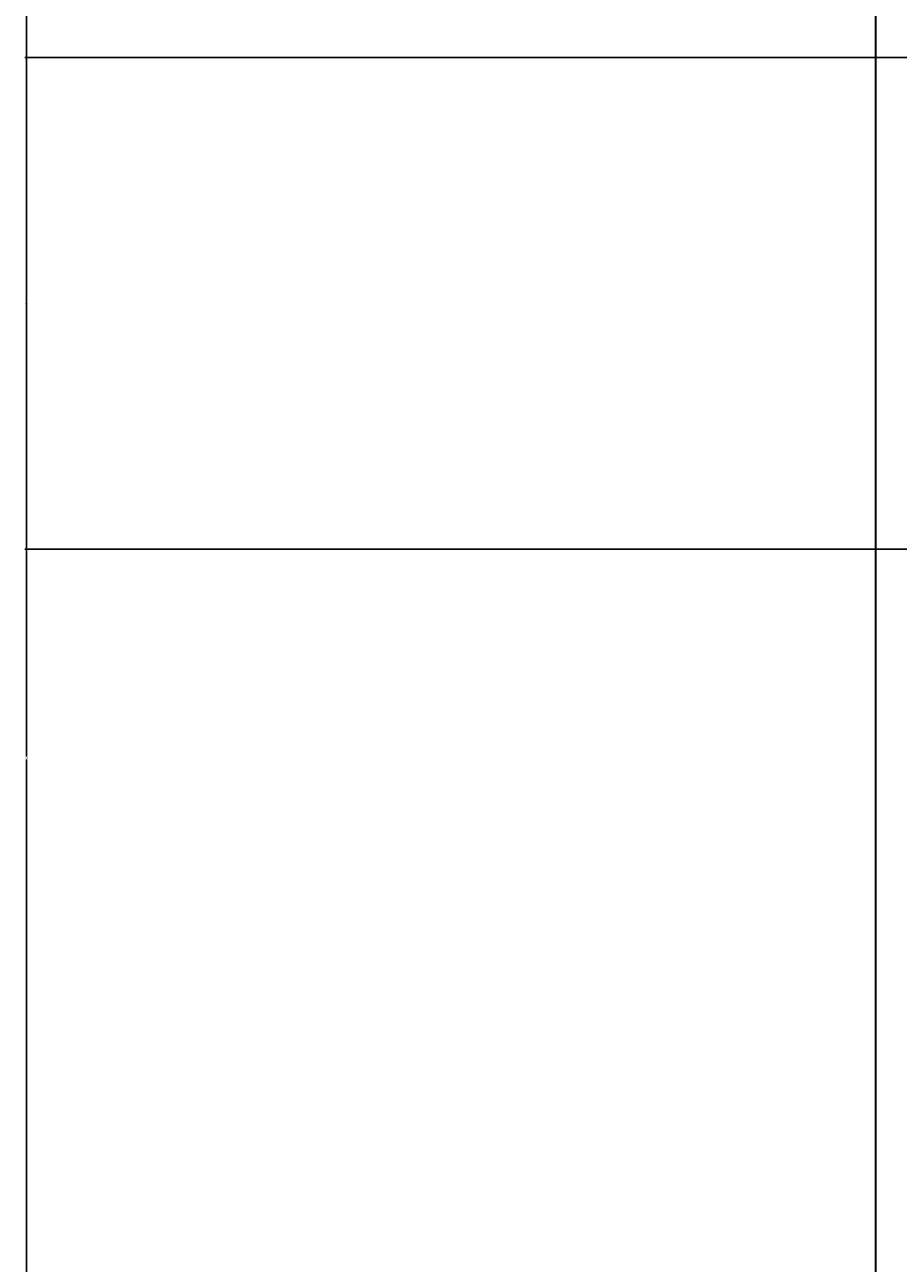
# Model space of a CAD drawing. Units: inches. Extents: x 3731 to 4318, y 1310 to 2388.
# Tile 24 of 57: x 3731 to 3838, y 1787 to 1938. Entities that reach past the tile are written whole.
import ezdxf

# ---------------------------------------------------------------- set-up
doc = ezdxf.new("R2010")
doc.units = ezdxf.units.IN
doc.layers.add('A-ANNO-DIMS', color=2, linetype='Continuous', lineweight=18)
doc.layers.add('A-WALL', color=7, linetype='Continuous', lineweight=35)
doc.styles.get("Standard").update_dxf_attribs({"font": 'arial.ttf'})
doc.dimstyles.get("Standard").update_dxf_attribs({"dimtxt": 0.18, "dimasz": 0.18, "dimexe": 0.18, "dimexo": 0.0625, "dimgap": 0.09, "dimtad": 0, "dimtih": 1, "dimtoh": 1, "dimdec": 4, "dimzin": 0, "dimdsep": 46, "dimtxsty": 'Standard', "dimcen": 0.09, "dimadec": 0, "dimazin": 0, "dimtfac": 1, "dimtdec": 4, "dimtofl": 0, "dimtmove": 0, "dimatfit": 3, "dimfxl": 1, "dimtolj": 1, "dimtzin": 0, "dimarcsym": 0})

# ---------------------------------------------------------------- blocks, each defined once
blk = doc.blocks.new('*D33')
at = {"layer": 'A-ANNO-DIMS', "color": 0, "lineweight": -2, "transparency": 16777216}
for p, q in [((3835.15, 2338.38), (3731.41, 2338.38)), ((3731.59, 2338.2), (3731.59, 1849.06)), ((3731.59, 1359.56), (3731.59, 1848.7)), ((3835.15, 1359.38), (3731.41, 1359.38))]:
    blk.add_line(p, q, dxfattribs=at)
at = {"layer": 'A-ANNO-DIMS', "color": 0, "transparency": 16777216}
for points in [[(3731.56, 2338.2), (3731.62, 2338.2), (3731.59, 2338.38)], [(3731.56, 1359.56), (3731.62, 1359.56), (3731.59, 1359.38)]]:
    blk.add_solid(points, dxfattribs=at)
at = {"layer": 'Defpoints', "color": 0, "transparency": 16777216}
for p in [(3731.59, 2338.38), (3835.21, 2338.38), (3835.21, 1359.38)]:
    blk.add_point(p, dxfattribs=at)
at = {"layer": 'A-ANNO-DIMS', "color": 0, "transparency": 16777216, "insert": (3731.59, 1848.88), "char_height": 0.18, "attachment_point": 5}
blk.add_mtext('\\A1;979', dxfattribs=at)
blk = doc.blocks.new('*D45')
at = {"layer": 'A-ANNO-DIMS', "color": 0, "lineweight": -2, "transparency": 16777216}
for p, q in [((3969.15, 1934.38), (3731.41, 1934.38)), ((3731.59, 1934.2), (3731.59, 1904.56)), ((3731.59, 1874.56), (3731.59, 1904.2)), ((3969.15, 1874.38), (3731.41, 1874.38))]:
    blk.add_line(p, q, dxfattribs=at)
at = {"layer": 'A-ANNO-DIMS', "color": 0, "transparency": 16777216}
for points in [[(3731.56, 1934.2), (3731.62, 1934.2), (3731.59, 1934.38)], [(3731.56, 1874.56), (3731.62, 1874.56), (3731.59, 1874.38)]]:
    blk.add_solid(points, dxfattribs=at)
at = {"layer": 'Defpoints', "color": 0, "transparency": 16777216}
for p in [(3731.59, 1934.38), (3969.21, 1934.38), (3969.21, 1874.38)]:
    blk.add_point(p, dxfattribs=at)
at = {"layer": 'A-ANNO-DIMS', "color": 0, "transparency": 16777216, "insert": (3731.59, 1904.38), "char_height": 0.18, "attachment_point": 5}
blk.add_mtext('\\A1;60', dxfattribs=at)

msp = doc.modelspace()

# ---------------------------------------------------------------- linework, layer by layer
at = {"layer": 'A-WALL'}
msp.add_line((3835.21, 2338.38), (3835.21, 1359.38), dxfattribs=at)

# ---------------------------------------------------------------- dimensions: what is measured, and where the dimension line sits
at = {"layer": 'A-ANNO-DIMS'}
for base, p1, p2, picture, middle in [((3731.59, 2338.38), (3835.21, 1359.38), (3835.21, 2338.38), '*D33', (3731.59, 1848.88)), ((3731.59, 1934.38), (3969.21, 1874.38), (3969.21, 1934.38), '*D45', (3731.59, 1904.38))]:
    dim = msp.add_linear_dim(base=base, p1=p1, p2=p2, angle=90, dimstyle='Standard', override={"dimdec": 0, "dimlfac": 1, "dimrnd": 0, "dimzin": 0, "dimdsep": 46, "dimlunit": 2}, dxfattribs=at)
    dim.commit()
    dim.dimension.update_dxf_attribs({"geometry": picture, "text_midpoint": middle})

doc.saveas('drawing.dxf')
